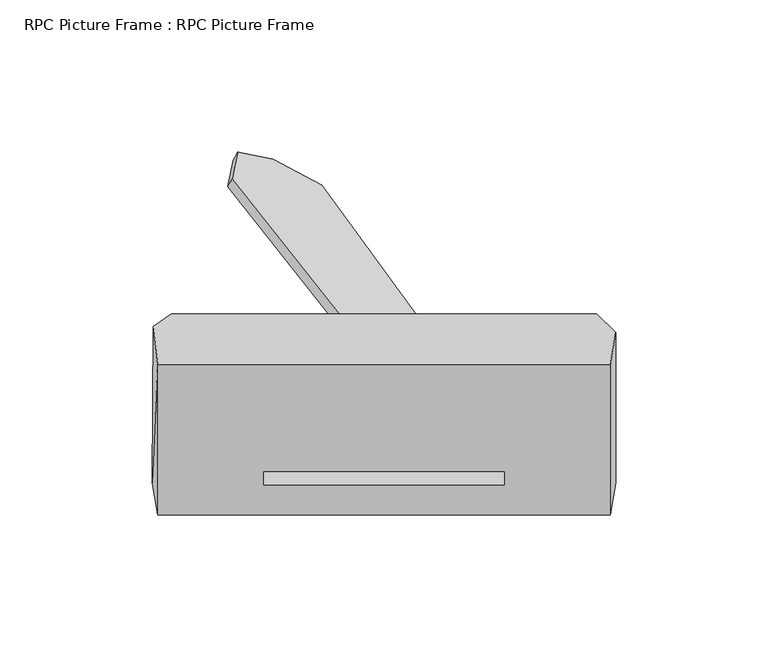
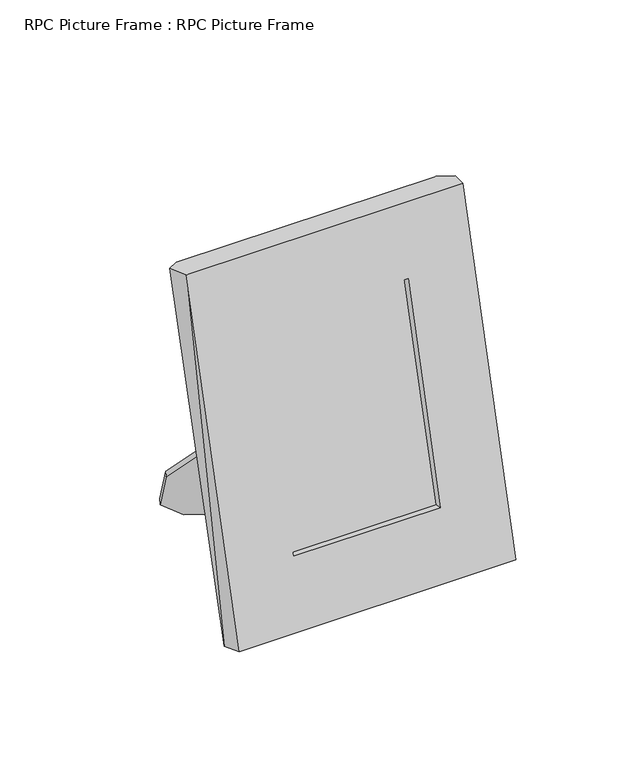
"""IFC4 building model written with IfcOpenShell, lengths in millimetres: proxy geometry, RPC Picture Frame : RPC Picture Frame."""

from ifc_helpers import new_model, si_unit, origin, place, context, project, spatial, triangles, source, transform, mapped, element, save


def rpc_picture_frame_rpc_picture_frame_c25e3fe9(model_context):
    return source(origin(), model_context, "Body", "Tessellation", [
        triangles([(31.2508246, -21.3381211, 97.8965409), (3.3584722, -15.6711751, 118.1948295), (-49.9194548, 51.6889462, 31.4618423), (-48.1092864, 60.5465677, 9.6660944), (-36.6253989, 58.2126713, 1.3093211), (-20.4915113, 49.7058959, 1.1720331), (29.8626917, -23.9491355, 96.7194234), (1.9728799, -18.2796482, 117.017712), (-51.3050488, 49.0855577, 30.2898095), (-49.492337, 57.9406358, 8.4915193), (-38.0084472, 55.6067394, 0.1347457), (-21.8771031, 47.0999685, -0.0025424), (74.3821513, -9.439824, 188.643936), (-74.3821513, -9.439824, 188.643936), (-75.8643555, 3.1347435, 185.2753007), (-69.9152047, 7.2228763, 184.1795282), (69.9152047, 7.2228763, 184.1795282), (76.2711348, 1.0830501, 185.8244496), (74.3821513, -58.7897891, 4.4644038), (-74.3821513, -58.8025018, 4.4440647), (-76.2711348, -48.2669167, 1.6449142), (-69.9152047, -42.1296323, 0.0), (69.9152047, -42.1296323, 0.0), (76.2711348, -48.2669167, 1.6449142), (39.7245466, -19.1135454, 152.5778598), (-39.7245466, -19.1135454, 152.5804032), (-39.7245466, -49.1364039, 40.5355663), (39.7245466, -49.1364039, 40.5355663), (39.7245466, -14.7203281, 151.4007423), (-39.7245466, -14.7203281, 151.4007423), (-39.7245466, -44.7431901, 39.3584488), (39.7245466, -44.7431901, 39.3584488)], [[1, 2, 8], [1, 8, 7], [2, 3, 9], [2, 9, 8], [3, 4, 10], [3, 10, 9], [4, 5, 11], [4, 11, 10], [5, 6, 12], [5, 12, 11], [6, 1, 7], [6, 7, 12], [1, 3, 2], [6, 3, 1], [6, 4, 3], [5, 4, 6], [7, 8, 9], [12, 7, 9], [12, 9, 10], [11, 12, 10], [15, 17, 16], [14, 17, 15], [13, 17, 14], [18, 17, 13], [21, 22, 23], [20, 21, 23], [19, 20, 23], [24, 19, 23], [23, 22, 16], [16, 17, 23], [20, 19, 27], [27, 19, 28], [14, 25, 13], [26, 25, 14], [14, 20, 27], [27, 26, 14], [28, 19, 13], [13, 25, 28], [29, 32, 28], [28, 25, 29], [30, 29, 25], [25, 26, 30], [31, 30, 26], [26, 27, 31], [32, 31, 27], [27, 28, 32], [31, 32, 29], [30, 31, 29], [14, 15, 21], [14, 21, 20], [15, 16, 22], [15, 22, 21], [17, 18, 24], [17, 24, 23], [18, 13, 19], [18, 19, 24]]),
    ])


if __name__ == "__main__":
    model = new_model("IFC4")
    model_context = context("Model", 3, world=origin())
    ifc_project = project(units=[si_unit("LENGTHUNIT", "METRE", prefix="MILLI")], contexts=[model_context])
    site = spatial("IfcSite", under=ifc_project)
    building = spatial("IfcBuilding", under=site)
    placement = place(None, origin())
    rpc_picture_frame_rpc_picture_frame_shape = rpc_picture_frame_rpc_picture_frame_c25e3fe9(model_context)
    element("IfcBuildingElementProxy", 1, Name="RPC Picture Frame : RPC Picture Frame", ObjectType="RPC Picture Frame : RPC Picture Frame", at=placement, inside=building, context=model_context, shape_type="MappedRepresentation", body=[
        mapped(rpc_picture_frame_rpc_picture_frame_shape, transform((0.0, 0.0, 0.0), x_axis=(1.0, 0.0, 0.0), y_axis=(0.0, 1.0, 0.0), z_axis=(0.0, 0.0, 1.0))),
    ])
    save(model, "model.ifc")

# Revit data of these elements
# Type "RPC Picture Frame : RPC Picture Frame"
#   built-in parameter 1005198 = "{2, 15},{39, RPC-16-8M5E-0H3T-F0AH-3U0K-JLQ7-G28B-AU},{1, 0},{1, 0},{2, 19},{1, 8},{5, Color},{1, 0},{1, 0},{3, 0.8},{3, 0.8},{3, 0.8},{1, 8},{7, BBoxMin},{1, 0},{1, 0},{1, 0},{1, 0},{1, 0},{1, 8},{7, BBoxMax},{1, 0},{1, 0},{1, 0},{1, 0},{1, 0},{2, 11},{9, RPCTypeId},{1, 0},{1, 0},{39, RPC-16-8M5E-0H3T-F0AH-3U0K-JLQ7-G28B-AU},{1, 6},{14, RPCPlantHeight},{1, 0},{1, 0},{5, 0.625},{2, 11},{7, keyword},{1, 0},{1, 0},{33, :RPCs:Office Clutter:Geometry:RPC},{2, 11},{8, category},{1, 0},{1, 0},{14, Office Clutter},{2, 11},{12, LocalizedUID},{1, 0},{1, 0},{13, Picture Frame},{2, 14},{6, Height},{1, 0},{1, 0},{5, 0.625},{1, 2},{16, Cast Reflections},{1, 0},{1, 0},{1, 0},{1, 2},{8, Portrait},{1, 0},{1, 0},{1, 1},{1, 2},{5, Stand},{1, 0},{1, 0},{1, 1},{2, 11},{10, RPCL_Frame},{1, 0},{1, 0},{5, Frame},{1, 4},{14, Frame Material},{1, 0},{1, 0},{1, 0},{2, 11},{12, RPCL_Picture},{1, 0},{1, 0},{7, Picture},{2, 11},{15, Picture Preview},{1, 0},{1, 0},{65, __RPC:/object data/textures/object/Photo/Photo0/textures/Portrait},{2, 11},{17, i_Picture Preview},{1, 0},{1, 0},{0, },{1, 2},{18, Use Custom Picture},{1, 0},{1, 0},{1, 0},{2, 11},{17, Picture File Name},{1, 0},{1, 0},{0, },{21, assetlibrary_base.fbx},{1, 5},"
#   built-in parameter 1005195 = "RPC-16-8M5E-0H3T-F0AH-3U0K-JLQ7-G28B-AU"
#   Height = 0
